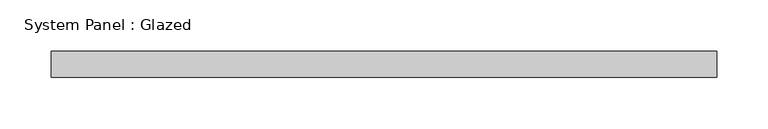
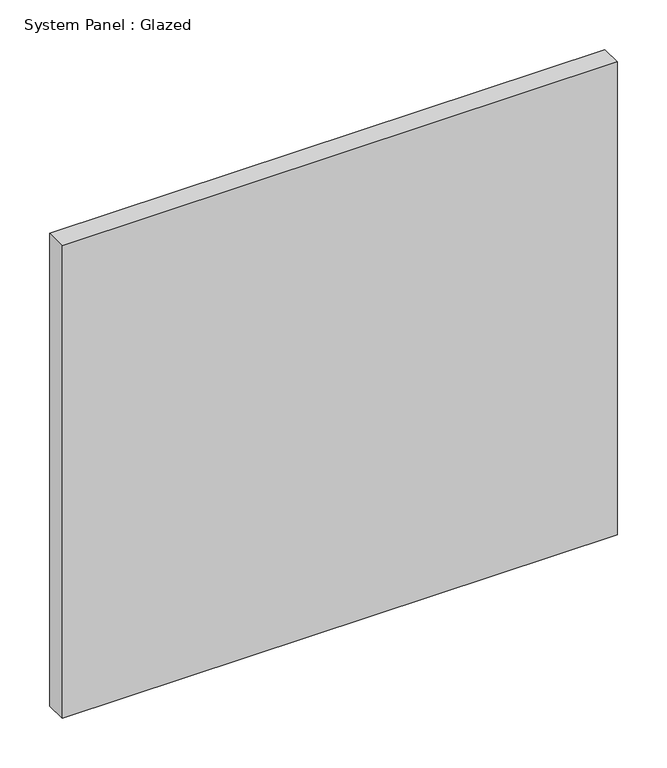
"""IFC4 building model written with IfcOpenShell, lengths in millimetres: plate geometry, System Panel : Glazed."""

from ifc_helpers import new_model, si_unit, origin, origin_with_axes, place, context, project, spatial, polyline, outline, extrude, source, transform, mapped, element, save


def system_panel_glazed_9fd70c8e(model_context):
    return source(origin(), model_context, "Body", "SweptSolid", [
        extrude(outline(polyline([(323.85, 19.05), (-323.85, 19.05), (-323.85, 44.45), (323.85, 44.45), (323.85, 19.05)])), origin_with_axes(), (0.0, 0.0, 1.0), 582.6996655),
    ])


if __name__ == "__main__":
    model = new_model("IFC4")
    model_context = context("Model", 3, world=origin())
    ifc_project = project(units=[si_unit("LENGTHUNIT", "METRE", prefix="MILLI")], contexts=[model_context])
    site = spatial("IfcSite", under=ifc_project)
    building = spatial("IfcBuilding", under=site)
    placement = place(None, origin())
    system_panel_glazed_shape = system_panel_glazed_9fd70c8e(model_context)
    element("IfcPlate", 1, ObjectType="System Panel : Glazed", at=placement, inside=building, context=model_context, shape_type="MappedRepresentation", body=[
        mapped(system_panel_glazed_shape, transform((0.0, 0.0, 0.0), x_axis=(1.0, 0.0, 0.0), y_axis=(0.0, 1.0, 0.0), z_axis=(0.0, 0.0, 1.0))),
    ])
    save(model, "model.ifc")

# Revit data of these elements
# Type "System Panel : Glazed"
#   Construction Type Id = "GSP4R"
#   Analytic Construction = "1/8 in Pilkington single glazing"
#   Visual Light Transmittance = 0.9
#   Solar Heat Gain Coefficient = 0.86
#   Heat Transfer Coefficient (U) = 1.18115 BTU/(h·ft²·°F)
#   Define Thermal Properties by = 1
# Element 1 (IfcPlate, "System Panel : Glazed")
#   Materials on its faces: "Glass"
# Materials
#   "Glass": class "Glass", colour RGB 0 128 192, transparency 0.75, Description = "Soda Lime Glass", Cost = 0
